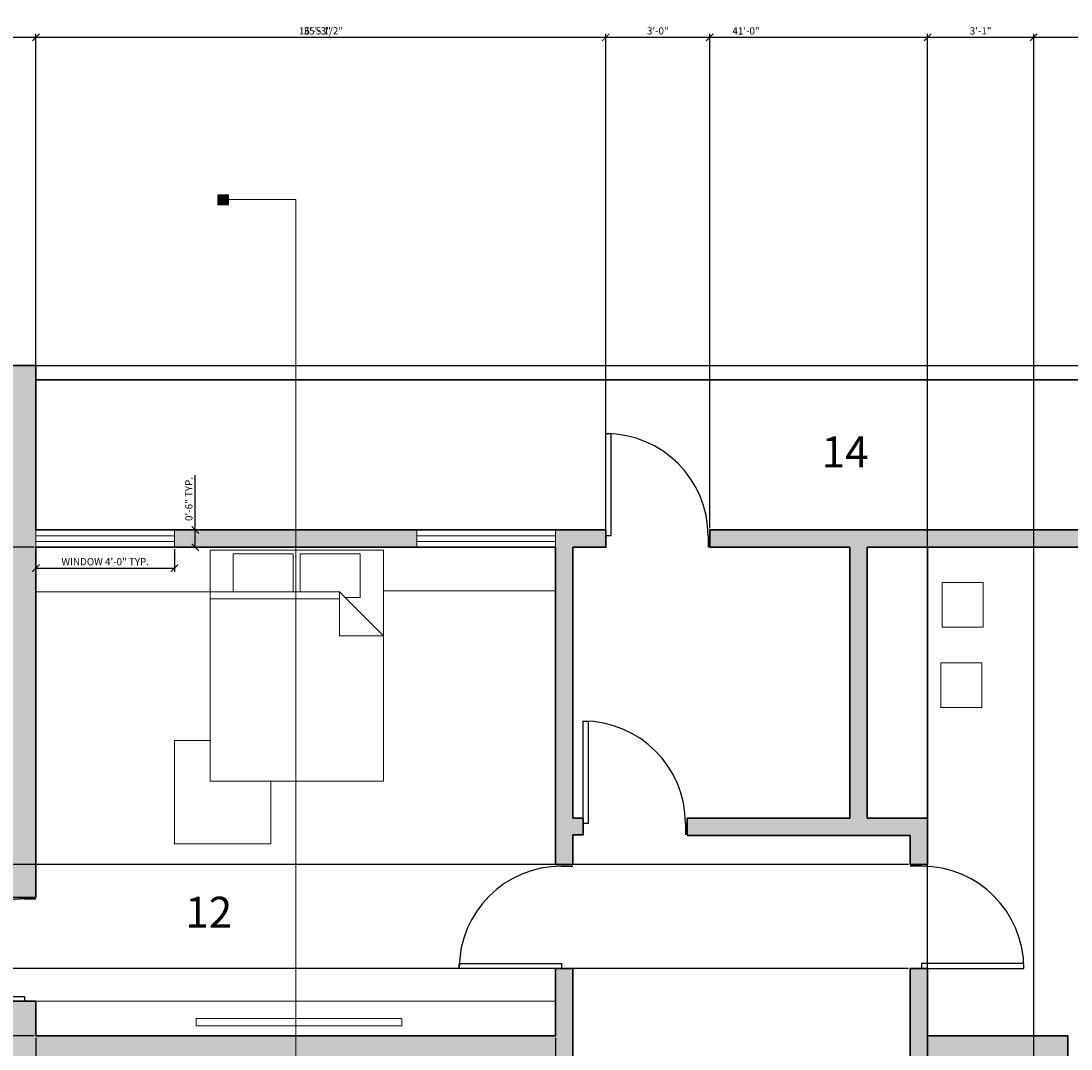
# Model space of a CAD drawing. Units: inches. Extents: x 3122 to 5933, y 1474 to 2995.
# Tile 9 of 12: x 5174 to 5538, y 2639 to 2995. Entities that reach past the tile are written whole.
import ezdxf

# ---------------------------------------------------------------- set-up
doc = ezdxf.new("R2010")
doc.units = ezdxf.units.IN
for name, color, linetype, lineweight in [('A-ANNO-DIMS', 2, 'Continuous', 18), ('A-ANNO-SYMB', 6, 'Continuous', 18), ('A-AREA-IDEN', 7, 'Continuous', 20), ('A-DOOR', 4, 'Continuous', 25), ('A-FLOR-CASE', 8, 'Continuous', 18), ('A-FURN', 8, 'Continuous', 18), ('A-GLAZ', 4, 'Continuous', 18), ('A-WALL', 7, 'Continuous', 35), ('A-WALL-PATT', 7, 'Continuous', 13), ('C-PROP', 7, 'Continuous', 25)]:
    doc.layers.add(name, color=color, linetype=linetype, lineweight=lineweight)
doc.styles.get("Standard").update_dxf_attribs({"font": 'arial.ttf'})
doc.dimstyles.new('ISO-25', dxfattribs={"dimtxt": 2.5, "dimasz": 2.5, "dimexe": 1.25, "dimexo": 0.625, "dimtad": 1, "dimdec": 0, "dimlunit": 3, "dimtxsty": 'Standard', "dimblk": 'ARCHTICK', "dimcen": 2.5, "dimadec": 0, "dimazin": 0, "dimtfac": 1, "dimtdec": 0, "dimtmove": 0, "dimatfit": 3, "dimfxl": 1, "dimarcsym": 0})

# ---------------------------------------------------------------- blocks, each defined once
blk = doc.blocks.new('*U25')
for p, q in [((0, 0), (0, -100)), ((900, 0), (900, -100))]:
    blk.add_line(p, q)
blk.add_lwpolyline([(0, 0), (0, 900), (43.75, 900), (43.75, 0)], close=True)
blk.add_arc((0, 0), 900, 0, 90)
blk = doc.blocks.new('*U27')
for p, q in [((0, 0), (0, 100)), ((900, 0), (900, 100))]:
    blk.add_line(p, q)
blk.add_lwpolyline([(0, 0), (0, -900), (43.75, -900), (43.75, 0)], close=True)
blk.add_arc((0, 0), 900, 270, 0)
blk = doc.blocks.new('Bed - Queen')
for p, q in [((0, -80.00003), (0, 0)), ((0, 0), (59.99999, 0)), ((59.99999, 0), (59.99999, -80.00003)), ((7.99999, -1.2), (28.79998, -1.2)), ((7.99999, -14.4), (7.99999, -1.2)), ((28.79998, -1.2), (28.79998, -14.4)), ((31.19999, -1.2), (51.99999, -1.2)), ((31.19999, -14.4), (31.19999, -1.2)), ((51.99999, -1.2), (51.99999, -16.4)), ((0, -14.4), (44.8, -14.4)), ((59.99999, -29.6), (44.8, -14.4)), ((44.8, -14.4), (44.8, -29.6)), ((44.8, -16.8), (0, -16.8)), ((51.99999, -16.4), (46.79936, -16.4)), ((44.8, -29.6), (59.99999, -29.6)), ((59.99999, -80.00003), (0, -80.00003))]:
    blk.add_line(p, q)
blk = doc.blocks.new('WIN-48-DOUBLE-LINE')
for p, q in [((0, 0), (0, 6)), ((48, 4), (0, 4)), ((48, 0), (48, 6)), ((48, 2), (0, 2))]:
    blk.add_line(p, q)
blk = doc.blocks.new('SECTION-LINE-END-MARK')
h = blk.add_hatch(color=256)
h.dxf.hatch_style = 1
h.paths.add_polyline_path([(3.68, 3.54), (0, 3.54), (0, 0), (3.68, 0)])
blk.add_lwpolyline([(0, 3.54), (3.68, 3.54), (3.68, 0), (0, 0)], close=True)
blk = doc.blocks.new('_ArchTick')
at = {"color": 0, "linetype": 'ByBlock', "const_width": 0.15}
blk.add_lwpolyline([(-0.5, -0.5), (0.5, 0.5)], dxfattribs=at)
blk = doc.blocks.new('*D72')
at = {"layer": 'A-ANNO-DIMS', "color": 0, "lineweight": -2, "transparency": 16777216}
for p, q in [((5178.96, 2812.27), (5178.96, 2804.45)), ((5226.96, 2812.27), (5226.96, 2804.45)), ((5178.96, 2805.7), (5226.96, 2805.7))]:
    blk.add_line(p, q, dxfattribs=at)
at = {"layer": 'Defpoints', "color": 0, "transparency": 16777216}
for p in [(5178.96, 2812.9), (5226.96, 2812.9), (5226.96, 2805.7)]:
    blk.add_point(p, dxfattribs=at)
at = {"layer": 'A-ANNO-DIMS', "color": 0, "lineweight": -2, "transparency": 16777216, "xscale": 2.5, "yscale": 2.5, "zscale": 2.5, "rotation": 180}
blk.add_blockref('_ArchTick', (5178.96, 2805.7), dxfattribs=at)
at = {"layer": 'A-ANNO-DIMS', "color": 0, "lineweight": -2, "transparency": 16777216, "xscale": 2.5, "yscale": 2.5, "zscale": 2.5}
blk.add_blockref('_ArchTick', (5226.96, 2805.7), dxfattribs=at)
at = {"layer": 'A-ANNO-DIMS', "color": 0, "transparency": 16777216, "insert": (5202.96, 2807.61), "char_height": 2.5, "attachment_point": 5}
blk.add_mtext('WINDOW 4\'-0" TYP.', dxfattribs=at)
blk = doc.blocks.new('*D73')
at = {"layer": 'A-ANNO-DIMS', "color": 0, "lineweight": -2, "transparency": 16777216}
for p, q in [((5234.16, 2818.9), (5234.16, 2837.88)), ((5227.59, 2818.9), (5235.41, 2818.9)), ((5234.16, 2812.9), (5234.16, 2818.9)), ((5227.59, 2812.9), (5235.41, 2812.9))]:
    blk.add_line(p, q, dxfattribs=at)
at = {"layer": 'Defpoints', "color": 0, "transparency": 16777216}
for p in [(5226.96, 2818.9), (5234.16, 2818.9), (5226.96, 2812.9)]:
    blk.add_point(p, dxfattribs=at)
at = {"layer": 'A-ANNO-DIMS', "color": 0, "lineweight": -2, "transparency": 16777216, "xscale": 2.5, "yscale": 2.5, "zscale": 2.5}
for p, rotation in [((5234.16, 2818.9), 90), ((5234.16, 2812.9), 270)]:
    blk.add_blockref('_ArchTick', p, dxfattribs=dict(at, rotation=rotation))
at = {"layer": 'A-ANNO-DIMS', "color": 0, "transparency": 16777216, "insert": (5232.26, 2829.64), "char_height": 2.5, "attachment_point": 5, "rotation": 90}
blk.add_mtext('0\'-6" TYP.', dxfattribs=at)
blk = doc.blocks.new('*D94')
at = {"layer": 'A-ANNO-DIMS', "color": 0, "lineweight": -2, "transparency": 16777216}
for p, q in [((5064.96, 1916.52), (5064.96, 2990.75)), ((5487.87, 1916.52), (5487.87, 2990.75)), ((5064.96, 2989.5), (5487.87, 2989.5))]:
    blk.add_line(p, q, dxfattribs=at)
at = {"layer": 'Defpoints', "color": 0, "transparency": 16777216}
for p in [(5487.87, 2989.5), (5064.96, 1915.9), (5487.87, 1915.9)]:
    blk.add_point(p, dxfattribs=at)
at = {"layer": 'A-ANNO-DIMS', "color": 0, "lineweight": -2, "transparency": 16777216, "xscale": 2.5, "yscale": 2.5, "zscale": 2.5, "rotation": 180}
blk.add_blockref('_ArchTick', (5064.96, 2989.5), dxfattribs=at)
at = {"layer": 'A-ANNO-DIMS', "color": 0, "lineweight": -2, "transparency": 16777216, "xscale": 2.5, "yscale": 2.5, "zscale": 2.5}
blk.add_blockref('_ArchTick', (5487.87, 2989.5), dxfattribs=at)
at = {"layer": 'A-ANNO-DIMS', "color": 0, "transparency": 16777216, "insert": (5276.42, 2991.41), "char_height": 2.5, "attachment_point": 5}
blk.add_mtext('35\'-3"', dxfattribs=at)
blk = doc.blocks.new('*D95')
at = {"layer": 'A-ANNO-DIMS', "color": 0, "lineweight": -2, "transparency": 16777216}
for p, q in [((5064.96, 2876.52), (5064.96, 2990.75)), ((5178.96, 2876.52), (5178.96, 2990.75)), ((5064.96, 2989.5), (5178.96, 2989.5))]:
    blk.add_line(p, q, dxfattribs=at)
at = {"layer": 'Defpoints', "color": 0, "transparency": 16777216}
for p in [(5178.96, 2989.5), (5064.96, 2875.9), (5178.96, 2875.9)]:
    blk.add_point(p, dxfattribs=at)
at = {"layer": 'A-ANNO-DIMS', "color": 0, "lineweight": -2, "transparency": 16777216, "xscale": 2.5, "yscale": 2.5, "zscale": 2.5, "rotation": 180}
blk.add_blockref('_ArchTick', (5064.96, 2989.5), dxfattribs=at)
at = {"layer": 'A-ANNO-DIMS', "color": 0, "lineweight": -2, "transparency": 16777216, "xscale": 2.5, "yscale": 2.5, "zscale": 2.5}
blk.add_blockref('_ArchTick', (5178.96, 2989.5), dxfattribs=at)
at = {"layer": 'A-ANNO-DIMS', "color": 0, "transparency": 16777216, "insert": (5121.96, 2991.4), "char_height": 2.5, "attachment_point": 5}
blk.add_mtext('9\'-6"', dxfattribs=at)
blk = doc.blocks.new('*D96')
at = {"layer": 'A-ANNO-DIMS', "color": 0, "lineweight": -2, "transparency": 16777216}
for p, q in [((5178.96, 2876.52), (5178.96, 2990.75)), ((5670.96, 2876.52), (5670.96, 2990.75)), ((5178.96, 2989.5), (5670.96, 2989.5))]:
    blk.add_line(p, q, dxfattribs=at)
at = {"layer": 'Defpoints', "color": 0, "transparency": 16777216}
for p in [(5670.96, 2989.5), (5178.96, 2875.9), (5670.96, 2875.9)]:
    blk.add_point(p, dxfattribs=at)
at = {"layer": 'A-ANNO-DIMS', "color": 0, "lineweight": -2, "transparency": 16777216, "xscale": 2.5, "yscale": 2.5, "zscale": 2.5, "rotation": 180}
blk.add_blockref('_ArchTick', (5178.96, 2989.5), dxfattribs=at)
at = {"layer": 'A-ANNO-DIMS', "color": 0, "lineweight": -2, "transparency": 16777216, "xscale": 2.5, "yscale": 2.5, "zscale": 2.5}
blk.add_blockref('_ArchTick', (5670.96, 2989.5), dxfattribs=at)
at = {"layer": 'A-ANNO-DIMS', "color": 0, "transparency": 16777216, "insert": (5424.96, 2991.4), "char_height": 2.5, "attachment_point": 5}
blk.add_mtext('41\'-0"', dxfattribs=at)
blk = doc.blocks.new('*D108')
at = {"layer": 'A-ANNO-DIMS', "color": 0, "lineweight": -2, "transparency": 16777216}
for p, q in [((5178.96, 2643.06), (5178.96, 1792.93)), ((5358.96, 2643.06), (5358.96, 1792.93)), ((5178.96, 1794.18), (5358.96, 1794.18))]:
    blk.add_line(p, q, dxfattribs=at)
at = {"layer": 'Defpoints', "color": 0, "transparency": 16777216}
for p in [(5178.96, 2643.69), (5358.96, 2643.69), (5358.96, 1794.18)]:
    blk.add_point(p, dxfattribs=at)
at = {"layer": 'A-ANNO-DIMS', "color": 0, "lineweight": -2, "transparency": 16777216, "xscale": 2.5, "yscale": 2.5, "zscale": 2.5, "rotation": 180}
blk.add_blockref('_ArchTick', (5178.96, 1794.18), dxfattribs=at)
at = {"layer": 'A-ANNO-DIMS', "color": 0, "lineweight": -2, "transparency": 16777216, "xscale": 2.5, "yscale": 2.5, "zscale": 2.5}
blk.add_blockref('_ArchTick', (5358.96, 1794.18), dxfattribs=at)
at = {"layer": 'A-ANNO-DIMS', "color": 0, "transparency": 16777216, "insert": (5268.96, 1796.08), "char_height": 2.5, "attachment_point": 5}
blk.add_mtext('15\'-0"', dxfattribs=at)
blk = doc.blocks.new('*D109')
at = {"layer": 'A-ANNO-DIMS', "color": 0, "lineweight": -2, "transparency": 16777216}
for p, q in [((5178.34, 2812.9), (4920.36, 2812.9)), ((4921.61, 2643.69), (4921.61, 2812.9)), ((5178.34, 2643.69), (4920.36, 2643.69))]:
    blk.add_line(p, q, dxfattribs=at)
at = {"layer": 'Defpoints', "color": 0, "transparency": 16777216}
for p in [(4921.61, 2812.9), (5178.96, 2812.9), (5178.96, 2643.69)]:
    blk.add_point(p, dxfattribs=at)
at = {"layer": 'A-ANNO-DIMS', "color": 0, "lineweight": -2, "transparency": 16777216, "xscale": 2.5, "yscale": 2.5, "zscale": 2.5}
for p, rotation in [((4921.61, 2812.9), 90), ((4921.61, 2643.69), 270)]:
    blk.add_blockref('_ArchTick', p, dxfattribs=dict(at, rotation=rotation))
at = {"layer": 'A-ANNO-DIMS', "color": 0, "transparency": 16777216, "insert": (4919.73, 2728.29), "char_height": 2.5, "attachment_point": 5, "rotation": 90}
blk.add_mtext('14\'-1"', dxfattribs=at)
blk = doc.blocks.new('*D110')
at = {"layer": 'A-ANNO-DIMS', "color": 0, "lineweight": -2, "transparency": 16777216}
for p, q in [((5487.87, 2643.06), (5487.87, 1792.93)), ((5670.96, 2643.06), (5670.96, 1792.93)), ((5487.87, 1794.18), (5670.96, 1794.18))]:
    blk.add_line(p, q, dxfattribs=at)
at = {"layer": 'Defpoints', "color": 0, "transparency": 16777216}
for p in [(5487.87, 2643.69), (5670.96, 2643.69), (5670.96, 1794.18)]:
    blk.add_point(p, dxfattribs=at)
at = {"layer": 'A-ANNO-DIMS', "color": 0, "lineweight": -2, "transparency": 16777216, "xscale": 2.5, "yscale": 2.5, "zscale": 2.5, "rotation": 180}
blk.add_blockref('_ArchTick', (5487.87, 1794.18), dxfattribs=at)
at = {"layer": 'A-ANNO-DIMS', "color": 0, "lineweight": -2, "transparency": 16777216, "xscale": 2.5, "yscale": 2.5, "zscale": 2.5}
blk.add_blockref('_ArchTick', (5670.96, 1794.18), dxfattribs=at)
at = {"layer": 'A-ANNO-DIMS', "color": 0, "transparency": 16777216, "insert": (5579.42, 1796.09), "char_height": 2.5, "attachment_point": 5}
blk.add_mtext('15\'-3"', dxfattribs=at)
blk = doc.blocks.new('*D114')
at = {"layer": 'A-ANNO-DIMS', "color": 0, "lineweight": -2, "transparency": 16777216}
for p, q in [((5487.87, 2539.31), (5487.87, 2990.75)), ((5524.65, 2539.31), (5524.65, 2990.75)), ((5487.87, 2989.5), (5524.65, 2989.5))]:
    blk.add_line(p, q, dxfattribs=at)
at = {"layer": 'Defpoints', "color": 0, "transparency": 16777216}
for p in [(5524.65, 2989.5), (5487.87, 2538.69), (5524.65, 2538.69)]:
    blk.add_point(p, dxfattribs=at)
at = {"layer": 'A-ANNO-DIMS', "color": 0, "lineweight": -2, "transparency": 16777216, "xscale": 2.5, "yscale": 2.5, "zscale": 2.5, "rotation": 180}
blk.add_blockref('_ArchTick', (5487.87, 2989.5), dxfattribs=at)
at = {"layer": 'A-ANNO-DIMS', "color": 0, "lineweight": -2, "transparency": 16777216, "xscale": 2.5, "yscale": 2.5, "zscale": 2.5}
blk.add_blockref('_ArchTick', (5524.65, 2989.5), dxfattribs=at)
at = {"layer": 'A-ANNO-DIMS', "color": 0, "transparency": 16777216, "insert": (5506.26, 2991.41), "char_height": 2.5, "attachment_point": 5}
blk.add_mtext('3\'-1"', dxfattribs=at)
blk = doc.blocks.new('*D120')
at = {"layer": 'A-ANNO-DIMS', "color": 0, "lineweight": -2, "transparency": 16777216}
for p, q in [((5481.24, 2703.06), (4920.36, 2703.06)), ((4921.61, 2667.06), (4921.61, 2703.06)), ((5481.24, 2667.06), (4920.36, 2667.06))]:
    blk.add_line(p, q, dxfattribs=at)
at = {"layer": 'Defpoints', "color": 0, "transparency": 16777216}
for p in [(4921.61, 2703.06), (5481.87, 2703.06), (5481.87, 2667.06)]:
    blk.add_point(p, dxfattribs=at)
at = {"layer": 'A-ANNO-DIMS', "color": 0, "lineweight": -2, "transparency": 16777216, "xscale": 2.5, "yscale": 2.5, "zscale": 2.5}
for p, rotation in [((4921.61, 2703.06), 90), ((4921.61, 2667.06), 270)]:
    blk.add_blockref('_ArchTick', p, dxfattribs=dict(at, rotation=rotation))
at = {"layer": 'A-ANNO-DIMS', "color": 0, "transparency": 16777216, "insert": (4919.71, 2685.06), "char_height": 2.5, "attachment_point": 5, "rotation": 90}
blk.add_mtext('3\'-0"', dxfattribs=at)
blk = doc.blocks.new('*D121')
at = {"layer": 'A-ANNO-DIMS', "color": 0, "lineweight": -2, "transparency": 16777216}
for p, q in [((5178.96, 2819.52), (5178.96, 2990.75)), ((5376.4, 2819.52), (5376.4, 2990.75)), ((5178.96, 2989.5), (5376.4, 2989.5))]:
    blk.add_line(p, q, dxfattribs=at)
at = {"layer": 'Defpoints', "color": 0, "transparency": 16777216}
for p in [(5376.4, 2989.5), (5178.96, 2818.9), (5376.4, 2818.9)]:
    blk.add_point(p, dxfattribs=at)
at = {"layer": 'A-ANNO-DIMS', "color": 0, "lineweight": -2, "transparency": 16777216, "xscale": 2.5, "yscale": 2.5, "zscale": 2.5, "rotation": 180}
blk.add_blockref('_ArchTick', (5178.96, 2989.5), dxfattribs=at)
at = {"layer": 'A-ANNO-DIMS', "color": 0, "lineweight": -2, "transparency": 16777216, "xscale": 2.5, "yscale": 2.5, "zscale": 2.5}
blk.add_blockref('_ArchTick', (5376.4, 2989.5), dxfattribs=at)
at = {"layer": 'A-ANNO-DIMS', "color": 0, "transparency": 16777216, "insert": (5277.68, 2991.42), "char_height": 2.5, "attachment_point": 5}
blk.add_mtext('16\'-5 1/2"', dxfattribs=at)
blk = doc.blocks.new('*D122')
at = {"layer": 'A-ANNO-DIMS', "color": 0, "lineweight": -2, "transparency": 16777216}
for p, q in [((5376.4, 2819.52), (5376.4, 2990.75)), ((5412.4, 2819.52), (5412.4, 2990.75)), ((5376.4, 2989.5), (5412.4, 2989.5))]:
    blk.add_line(p, q, dxfattribs=at)
at = {"layer": 'Defpoints', "color": 0, "transparency": 16777216}
for p in [(5412.4, 2989.5), (5376.4, 2818.9), (5412.4, 2818.9)]:
    blk.add_point(p, dxfattribs=at)
at = {"layer": 'A-ANNO-DIMS', "color": 0, "lineweight": -2, "transparency": 16777216, "xscale": 2.5, "yscale": 2.5, "zscale": 2.5, "rotation": 180}
blk.add_blockref('_ArchTick', (5376.4, 2989.5), dxfattribs=at)
at = {"layer": 'A-ANNO-DIMS', "color": 0, "lineweight": -2, "transparency": 16777216, "xscale": 2.5, "yscale": 2.5, "zscale": 2.5}
blk.add_blockref('_ArchTick', (5412.4, 2989.5), dxfattribs=at)
at = {"layer": 'A-ANNO-DIMS', "color": 0, "transparency": 16777216, "insert": (5394.4, 2991.41), "char_height": 2.5, "attachment_point": 5}
blk.add_mtext('3\'-0"', dxfattribs=at)

msp = doc.modelspace()

# ---------------------------------------------------------------- hatches: boundary and pattern name
at = {"layer": 'A-WALL-PATT'}
h = msp.add_hatch(color=256, dxfattribs=at)
h.dxf.hatch_style = 1
h.paths.add_polyline_path([(5073.96, 2454.69), (5101.59, 2454.69), (5101.59, 2459.69), (5101.59, 2463.69), (5073.96, 2463.69), (5073.96, 2634.69), (5169.96, 2634.69), (5364.96, 2634.69), (5364.96, 2643.69), (5364.96, 2667.06), (5358.96, 2667.06), (5358.96, 2643.69), (5178.96, 2643.69), (5178.96, 2655.69), (5169.96, 2655.69), (5169.96, 2643.69), (5073.96, 2643.69), (5073.96, 2745.9), (5124.13, 2745.9), (5124.13, 2754.9), (5073.96, 2754.9), (5073.96, 2866.9), (5169.96, 2866.9), (5169.96, 2818.9), (5169.96, 2812.9), (5169.96, 2754.9), (5154.13, 2754.9), (5154.13, 2745.9), (5169.96, 2745.9), (5169.96, 2691.69), (5178.96, 2691.69), (5178.96, 2812.9), (5178.96, 2818.9), (5178.96, 2875.9), (5064.96, 2875.9), (5064.96, 2055.71), (5217.96, 2055.71), (5217.96, 2464.19), (5212.96, 2464.19), (5212.96, 2463.69), (5148.19, 2463.69), (5148.19, 2459.69), (5148.19, 2454.69), (5158.96, 2454.69), (5158.96, 2450.72), (5156.04, 2450.72), (5156.04, 2447.72), (5158.96, 2447.72), (5158.96, 2425.1), (5164.96, 2425.1), (5164.96, 2447.72), (5167.71, 2447.72), (5167.71, 2450.72), (5164.96, 2450.72), (5164.96, 2454.69), (5212.96, 2454.69), (5212.96, 2064.71), (5073.96, 2064.71), (5073.96, 2322.69), (5158.96, 2322.69), (5164.96, 2322.69), (5164.96, 2328.69), (5158.96, 2328.69), (5073.96, 2328.69)])
h = msp.add_hatch(color=256, dxfattribs=at)
h.dxf.hatch_style = 1
h.paths.add_polyline_path([(5536.42, 2643.69), (5487.87, 2643.69), (5487.87, 2667.06), (5485.81, 2667.06), (5481.87, 2667.06), (5481.87, 2643.69), (5481.87, 2590.35), (5487.87, 2590.35), (5487.87, 2634.69), (5524.65, 2634.69), (5524.65, 2538.69), (5487.87, 2538.69), (5487.87, 2554.35), (5481.87, 2554.35), (5481.87, 2532.69), (5524.65, 2532.69), (5658.65, 2532.69), (5718.65, 2532.69), (5718.65, 2501.93), (5724.65, 2501.93), (5724.65, 2549.4), (5718.65, 2549.4), (5718.65, 2538.69), (5658.65, 2538.69), (5658.65, 2573.57), (5658.59, 2573.63), (5654.65, 2573.63), (5654.65, 2538.69), (5594.65, 2538.69), (5594.65, 2573.57), (5594.59, 2573.63), (5590.65, 2573.63), (5590.65, 2538.69), (5530.65, 2538.69), (5530.65, 2634.69), (5536.42, 2634.69)])
h.paths.add_polyline_path([(5735.69, 2643.69), (5679.96, 2643.69), (5679.96, 2710.77), (5720.44, 2710.77), (5720.44, 2687.32), (5737.79, 2687.32), (5737.79, 2692.32), (5725.44, 2692.32), (5725.44, 2715.77), (5679.96, 2715.77), (5679.96, 2866.9), (5775.96, 2866.9), (5775.96, 2692.32), (5773.79, 2692.32), (5773.79, 2687.32), (5775.96, 2687.32), (5775.96, 2643.69), (5775.96, 2591.85), (5784.96, 2591.85), (5784.96, 2875.9), (5670.96, 2875.9), (5670.96, 2818.9), (5412.4, 2818.9), (5412.4, 2812.9), (5460.96, 2812.9), (5460.96, 2719.12), (5404.54, 2719.12), (5404.54, 2713.12), (5466.96, 2713.12), (5481.87, 2713.12), (5481.87, 2703.06), (5487.87, 2703.06), (5487.87, 2719.12), (5466.96, 2719.12), (5466.96, 2812.9), (5670.96, 2812.9), (5670.96, 2643.69), (5572.42, 2643.69), (5572.42, 2634.69), (5718.65, 2634.69), (5718.65, 2549.4), (5724.65, 2549.4), (5724.65, 2591.85), (5739.96, 2591.85), (5739.96, 2596.85), (5724.65, 2596.85), (5724.65, 2634.69), (5735.69, 2634.69)])
h.paths.add_polyline_path([(5594.65, 2634.69), (5590.65, 2634.69), (5590.65, 2603.63), (5594.65, 2603.63)], flags=17)
h.paths.add_polyline_path([(5724.65, 2441.93), (5718.65, 2441.93), (5718.65, 2336.51), (5724.65, 2336.51)])
h.paths.add_polyline_path([(5724.65, 2276.51), (5718.65, 2276.51), (5718.65, 2250.49), (5713.26, 2250.49), (5713.26, 2244.39), (5724.65, 2244.39)])
h.paths.add_polyline_path([(5689.26, 2250.49), (5540.87, 2250.49), (5540.87, 2317.46), (5535.87, 2317.46), (5535.87, 2244.39), (5689.26, 2244.39)])
h.paths.add_polyline_path([(5540.87, 2532.69), (5535.87, 2532.69), (5535.87, 2472.78), (5540.87, 2472.78)])
h.paths.add_polyline_path([(5540.87, 2472.78), (5537.87, 2472.78), (5537.87, 2346.69), (5537.87, 2317.46), (5540.87, 2317.46)])
h = msp.add_hatch(color=256, dxfattribs=at)
h.dxf.hatch_style = 1
h.paths.add_polyline_path([(5364.96, 2812.9), (5376.4, 2812.9), (5376.4, 2816.83), (5376.4, 2818.9), (5358.96, 2818.9), (5358.96, 2812.9), (5358.96, 2703.06), (5364.96, 2703.06), (5364.96, 2713.36), (5368.54, 2713.36), (5368.54, 2717.3), (5368.54, 2719.12), (5364.96, 2719.12)])
h.paths.add_polyline_path([(5310.96, 2818.9), (5226.96, 2818.9), (5226.96, 2812.9), (5310.96, 2812.9)])

# ---------------------------------------------------------------- linework, layer by layer
at = {"layer": 'A-ANNO-SYMB'}
for q in [(5245.58, 2933.31), (5268.96, 1850.37)]:
    msp.add_line((5268.96, 2933.31), q, dxfattribs=at)
at = {"layer": 'A-FLOR-CASE'}
for p, q in [((5299.3, 2797.81), (5358.96, 2797.81)), ((5239.31, 2797.5), (5178.96, 2797.5)), ((5239.31, 2746.06), (5226.97, 2746.06)), ((5226.97, 2746.06), (5226.97, 2710.18)), ((5260.3, 2710.18), (5260.3, 2731.9)), ((5226.97, 2710.18), (5260.3, 2710.18)), ((5178.96, 2655.69), (5358.96, 2655.69))]:
    msp.add_line(p, q, dxfattribs=at)
msp.add_lwpolyline([(5234.45, 2649.78), (5305.69, 2649.78), (5305.69, 2647.2), (5234.45, 2647.2)], close=True, dxfattribs=at)
at = {"layer": 'A-FURN'}
for points in [[(5492.89, 2800.77), (5507.15, 2800.77), (5507.15, 2785.24), (5492.89, 2785.24)], [(5492.41, 2772.92), (5506.66, 2772.92), (5506.66, 2757.39), (5492.41, 2757.39)]]:
    msp.add_lwpolyline(points, close=True, dxfattribs=at)
at = {"layer": 'A-GLAZ'}
for p, q in [((5226.96, 2816.9), (5178.96, 2816.9)), ((5226.96, 2814.9), (5178.96, 2814.9))]:
    msp.add_line(p, q, dxfattribs=at)
at = {"layer": 'A-WALL'}
for p, q in [((5178.96, 2875.9), (5064.96, 2875.9)), ((5178.96, 2875.9), (5178.96, 2818.9)), ((5178.96, 2870.9), (5670.96, 2870.9)), ((5376.4, 2818.9), (5178.96, 2818.9)), ((5376.4, 2812.9), (5376.4, 2818.9)), ((5670.96, 2818.9), (5412.4, 2818.9)), ((5412.4, 2812.9), (5412.4, 2818.9)), ((5178.96, 2812.9), (5178.96, 2691.69)), ((5358.96, 2812.9), (5178.96, 2812.9)), ((5358.96, 2812.9), (5358.96, 2703.06)), ((5364.96, 2812.9), (5364.96, 2719.12)), ((5376.4, 2812.9), (5364.96, 2812.9)), ((5460.96, 2812.9), (5412.4, 2812.9)), ((5460.96, 2812.9), (5460.96, 2719.12)), ((5670.96, 2812.9), (5466.96, 2812.9)), ((5466.96, 2812.9), (5466.96, 2719.12)), ((5487.87, 2719.12), (5487.87, 2812.9)), ((5368.54, 2719.12), (5364.96, 2719.12)), ((5368.54, 2713.36), (5368.54, 2719.12)), ((5404.54, 2713.36), (5404.54, 2719.12)), ((5404.54, 2719.12), (5460.96, 2719.12)), ((5466.96, 2719.12), (5487.87, 2719.12)), ((5487.87, 2719.12), (5487.87, 2703.06)), ((5364.96, 2713.36), (5368.54, 2713.36)), ((5364.96, 2713.36), (5364.96, 2703.06)), ((5404.54, 2713.12), (5466.96, 2713.12)), ((5466.96, 2713.12), (5481.87, 2713.12)), ((5481.87, 2713.12), (5481.87, 2703.06)), ((5358.96, 2703.06), (5364.96, 2703.06)), ((5481.87, 2703.06), (5487.87, 2703.06)), ((5169.96, 2691.69), (5178.96, 2691.69)), ((5358.96, 2667.06), (5364.96, 2667.06)), ((5358.96, 2667.06), (5358.96, 2643.69)), ((5364.96, 2667.06), (5364.96, 2643.69)), ((5481.87, 2667.06), (5487.87, 2667.06)), ((5481.87, 2667.06), (5481.87, 2643.69)), ((5487.87, 2667.06), (5487.87, 2643.69)), ((5169.96, 2655.69), (5178.96, 2655.69)), ((5178.96, 2655.69), (5178.96, 2643.69)), ((5178.96, 2643.69), (5358.96, 2643.69)), ((5364.96, 2643.69), (5364.96, 2634.69)), ((5481.87, 2643.69), (5481.87, 2532.69)), ((5487.87, 2643.69), (5536.42, 2643.69)), ((5536.42, 2643.69), (5536.42, 2634.69))]:
    msp.add_line(p, q, dxfattribs=at)
at = {"layer": 'C-PROP'}
msp.add_line((5178.96, 2875.9), (5670.96, 2875.9), dxfattribs=at)

# ---------------------------------------------------------------- block references
at = {"layer": 'A-ANNO-SYMB'}
msp.add_blockref('SECTION-LINE-END-MARK', (5241.93, 2931.46), dxfattribs=at)
at = {"layer": 'A-DOOR', "xscale": 0.0393700787401575, "yscale": 0.0393700787401575, "zscale": 0.0393700787401575}
for p in [(5376.4, 2816.83), (5368.54, 2717.3)]:
    msp.add_blockref('*U25', p, dxfattribs=at)
at = {"layer": 'A-DOOR', "xscale": 0.0393700787401575, "yscale": 0.0393700787401575, "zscale": 0.0393700787401575, "rotation": 90}
for name, p in [('*U25', (5361.03, 2667.06)), ('*U27', (5485.81, 2667.06)), ('*U25', (5175.03, 2655.69))]:
    msp.add_blockref(name, p, dxfattribs=at)
at = {"layer": 'A-FURN'}
msp.add_blockref('Bed - Queen', (5239.31, 2811.9), dxfattribs=at)
at = {"layer": 'A-GLAZ'}
for p in [(5178.96, 2812.9), (5310.96, 2812.9)]:
    msp.add_blockref('WIN-48-DOUBLE-LINE', p, dxfattribs=at)

# ---------------------------------------------------------------- texts
at = {"layer": 'A-AREA-IDEN'}
for s, p in [('14', (5451.18, 2840.56)), ('12', (5230.69, 2681.18))]:
    msp.add_text(s, height=10.725, rotation=0.0333, dxfattribs=at).set_placement(p)

# ---------------------------------------------------------------- dimensions: what is measured, and where the dimension line sits
at = {"layer": 'A-ANNO-DIMS'}
for base, p1, p2, picture, middle in [((5376.4, 2989.5), (5178.96, 2818.9), (5376.4, 2818.9), '*D121', (5277.68, 2991.42)), ((5487.87, 2989.5), (5064.96, 1915.9), (5487.87, 1915.9), '*D94', (5276.42, 2991.41)), ((5178.96, 2989.5), (5064.96, 2875.9), (5178.96, 2875.9), '*D95', (5121.96, 2991.4)), ((5670.96, 2989.5), (5178.96, 2875.9), (5670.96, 2875.9), '*D96', (5424.96, 2991.4)), ((5412.4, 2989.5), (5376.4, 2818.9), (5412.4, 2818.9), '*D122', (5394.4, 2991.41)), ((5524.65, 2989.5), (5487.87, 2538.69), (5524.65, 2538.69), '*D114', (5506.26, 2991.41)), ((5358.96, 1794.18), (5178.96, 2643.69), (5358.96, 2643.69), '*D108', (5268.96, 1796.08)), ((5670.96, 1794.18), (5487.87, 2643.69), (5670.96, 2643.69), '*D110', (5579.42, 1796.09))]:
    dim = msp.add_linear_dim(base=base, p1=p1, p2=p2, dimstyle='ISO-25', override={"dimdec": 1, "dimlfac": 1, "dimrnd": 0, "dimzin": 1, "dimdsep": 46, "dimlunit": 4, "dimfrac": 2}, dxfattribs=at)
    dim.commit()
    dim.dimension.update_dxf_attribs({"geometry": picture, "text_midpoint": middle})
dim = msp.add_linear_dim(base=(5234.16, 2818.9), p1=(5226.96, 2812.9), p2=(5226.96, 2818.9), angle=90, text='<> TYP.', dimstyle='ISO-25', override={"dimdec": 1, "dimlfac": 1, "dimrnd": 0, "dimzin": 1, "dimdsep": 46, "dimlunit": 4, "dimfrac": 2}, dxfattribs=at)
dim.commit()
dim.dimension.update_dxf_attribs({"geometry": '*D73', "text_midpoint": (5232.26, 2829.64)})
for base, p1, p2, picture, middle in [((4921.61, 2812.9), (5178.96, 2643.69), (5178.96, 2812.9), '*D109', (4919.73, 2728.29)), ((4921.61, 2703.06), (5481.87, 2667.06), (5481.87, 2703.06), '*D120', (4919.71, 2685.06))]:
    dim = msp.add_linear_dim(base=base, p1=p1, p2=p2, angle=90, dimstyle='ISO-25', override={"dimdec": 1, "dimlfac": 1, "dimrnd": 0, "dimzin": 1, "dimdsep": 46, "dimlunit": 4, "dimfrac": 2}, dxfattribs=at)
    dim.commit()
    dim.dimension.update_dxf_attribs({"geometry": picture, "text_midpoint": middle})
dim = msp.add_linear_dim(base=(5226.96, 2805.7), p1=(5178.96, 2812.9), p2=(5226.96, 2812.9), text='WINDOW <> TYP.', dimstyle='ISO-25', override={"dimdec": 1, "dimlfac": 1, "dimrnd": 0, "dimzin": 1, "dimdsep": 46, "dimlunit": 4, "dimfrac": 2}, dxfattribs=at)
dim.commit()
dim.dimension.update_dxf_attribs({"geometry": '*D72', "text_midpoint": (5202.96, 2807.61)})

doc.saveas('drawing.dxf')
